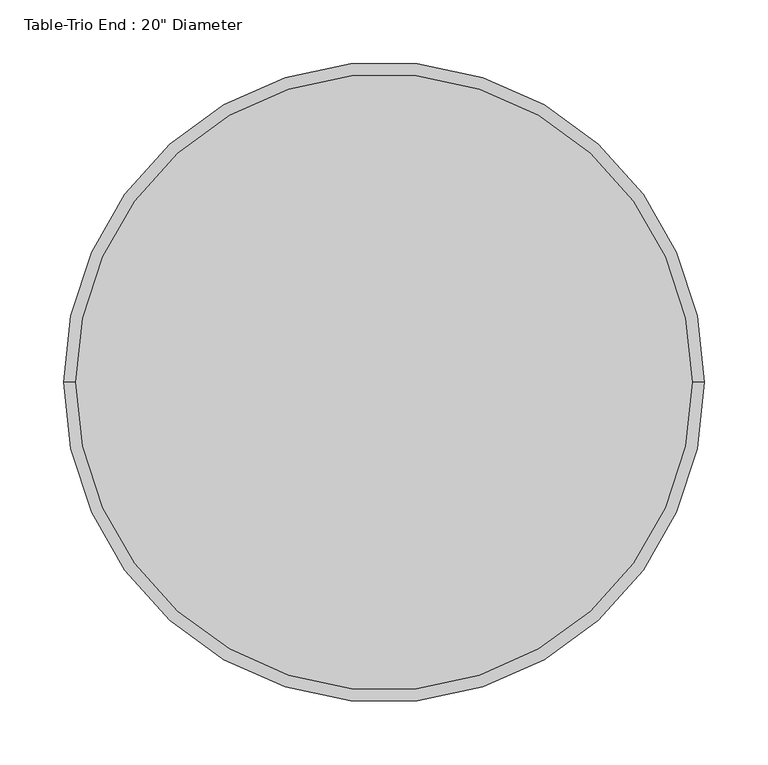
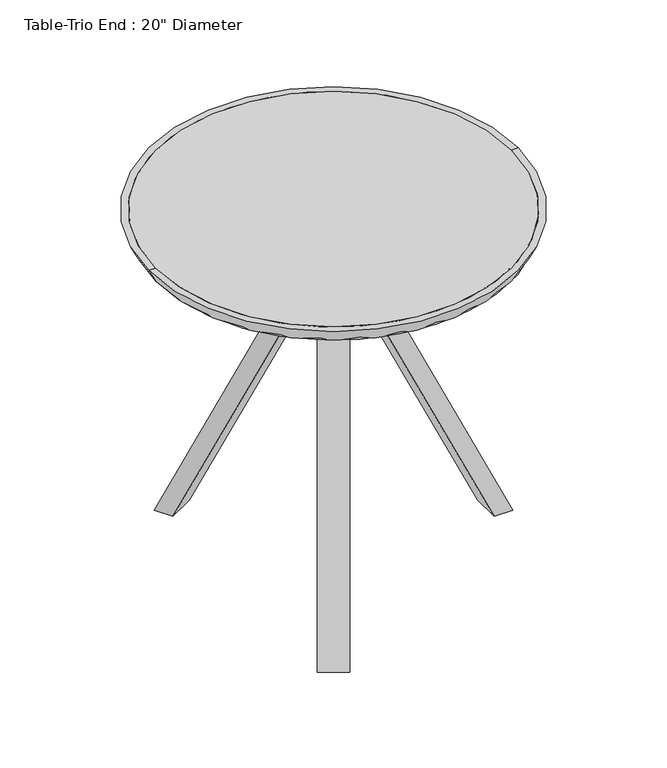
"""IFC4 building model written with IfcOpenShell, lengths in millimetres: furniture geometry."""

from ifc_helpers import new_model, si_unit, point, frame, frame_2d, origin, origin_2d, place, context, project, spatial, polyline, circle_curve, trimmed, segment, composite_curve, outline, extrude, source, transform, mapped, element, save
from ifc_brep_helpers import plane_surface, revolved_surface, advanced_brep


def furniture_9d41381f(model_context):
    return source(origin(), model_context, "Body", "SolidModel", [
        extrude(outline(composite_curve([segment(trimmed(circle_curve(origin_2d(), 241.3), [point((-241.3, 0.0))], [point((241.3, 0.0))], False, "CARTESIAN"), True, "CONTINUOUS"), segment(trimmed(circle_curve(origin_2d(), 241.3), [point((241.3, 0.0))], [point((-241.3, 0.0))], False, "CARTESIAN"), True, "CONTINUOUS")], self_intersect=False)), frame((0.0, 0.0, 482.6), z_axis=(0.0, 0.0, 1.0), x_axis=(1.0, 0.0, 0.0)), (0.0, 0.0, 1.0), 19.05),
        advanced_brep(
        [(241.3, 0.0, 482.6), (-241.3, 0.0, 482.6), (-241.3, 0.0, 501.65), (241.3, 0.0, 501.65), (250.825, 0.0, 501.65), (-250.825, 0.0, 501.65)],
        [
            (0, 1, circle_curve(frame((0.0, 0.0, 482.6), z_axis=(0.0, 0.0, -1.0), x_axis=(-1.0, 0.0, 0.0)), 241.3)),
            (1, 2),
            (2, 3, circle_curve(frame((0.0, 0.0, 501.65), z_axis=(0.0, 0.0, 1.0), x_axis=(-1.0, 0.0, 0.0)), 241.3)),
            (3, 0),
            (4, 5, circle_curve(frame((0.0, 0.0, 501.65), z_axis=(0.0, 0.0, -1.0), x_axis=(-1.0, 0.0, 0.0)), 250.825)),
            (5, 1),
            (0, 4),
            (2, 5),
            (4, 3),
            (1, 0, circle_curve(frame((0.0, 0.0, 482.6), z_axis=(0.0, 0.0, -1.0), x_axis=(1.0, 0.0, 0.0)), 241.3)),
            (3, 2, circle_curve(frame((0.0, 0.0, 501.65), z_axis=(0.0, 0.0, 1.0), x_axis=(1.0, 0.0, 0.0)), 241.3)),
            (5, 4, circle_curve(frame((0.0, 0.0, 501.65), z_axis=(0.0, 0.0, -1.0), x_axis=(1.0, 0.0, 0.0)), 250.825)),
        ],
        [
            revolved_surface(polyline([(-241.3, 0.0, 501.65), (-241.3, 0.0, 482.6)]), (0.0, 0.0, 0.0), (0.0, 0.0, 1.0)),
            revolved_surface(polyline([(-241.3, 0.0, 482.6), (-250.825, 0.0, 501.65)]), (0.0, 0.0, 0.0), (0.0, 0.0, 1.0)),
            plane_surface(frame((0.0, 0.0, 501.65), z_axis=(0.0, 0.0, 1.0), x_axis=(-1.0, 0.0, 0.0))),
            revolved_surface(polyline([(241.3, 0.0, 501.65), (241.3, 0.0, 482.6)]), (0.0, 0.0, 0.0), (0.0, 0.0, 1.0)),
            revolved_surface(polyline([(241.3, 0.0, 482.6), (250.825, 0.0, 501.65)]), (0.0, 0.0, 0.0), (0.0, 0.0, 1.0)),
            plane_surface(frame((0.0, 0.0, 501.65), z_axis=(0.0, 0.0, 1.0), x_axis=(1.0, 0.0, 0.0))),
        ],
        [
            (0, [[1, 2, 3, 4]]),
            (1, [[5, 6, -1, 7]]),
            (2, [[-3, 8, -5, 9]]),
            (3, [[10, -4, 11, -2]]),
            (4, [[12, -7, -10, -6]]),
            (5, [[-11, -9, -12, -8]]),
        ],
    ),
        extrude(outline(composite_curve([segment(polyline([(374.1964885, 32.5393466), (0.0, 207.0300348), (0.0, 232.3753669), (384.9309923, 52.8790974)]), True, "CONTINUOUS"), segment(trimmed(circle_curve(frame_2d((406.4, 98.9195329)), 50.8), [point((384.9309923, 52.8790974))], [point((457.2, 98.9195329))], True, "CARTESIAN"), True, "CONTINUOUS"), segment(polyline([(457.2, 98.9195329), (457.2, 154.8312035), (482.6, 154.8312035), (482.6, 101.6)]), True, "CONTINUOUS"), segment(trimmed(circle_curve(frame_2d((406.4, 101.6)), 76.2), [point((482.6, 101.6))], [point((374.1964885, 32.5393466))], False, "CARTESIAN"), True, "CONTINUOUS")], self_intersect=False)), frame((0.0, -19.05, 0.0), z_axis=(0.0, 1.0, 0.0), x_axis=(0.0, 0.0, 1.0)), (0.0, 0.0, 1.0), 38.1),
        extrude(outline(composite_curve([segment(trimmed(circle_curve(frame_2d((412.8801427, -76.2)), 76.2), [point((412.8801427, 0.0))], [point((481.9407961, -108.4035115))], False, "CARTESIAN"), True, "CONTINUOUS"), segment(polyline([(481.9407961, -108.4035115), (459.4443174, -156.6473658), (436.4240996, -145.9128619), (460.0533926, -95.2396796)]), True, "CONTINUOUS"), segment(trimmed(circle_curve(frame_2d((414.012957, -73.7706719)), 50.8), [point((460.0533926, -95.2396796))], [point((414.0129571, -22.9706718))], True, "CARTESIAN"), True, "CONTINUOUS"), segment(polyline([(414.0129571, -22.9706718), (-10.7114002, -22.9706719), (0.0, 0.0), (412.8801427, 0.0)]), True, "CONTINUOUS")], self_intersect=False)), frame((-120.0128014, 169.7682695, 0.0), z_axis=(0.8660254037844397, 0.4999999999999983, 0.0), x_axis=(0.2113091308703442, -0.36599815077065895, 0.9063077870366545)), (0.0, 0.0, 1.0), 38.1),
        extrude(outline(composite_curve([segment(trimmed(circle_curve(frame_2d((412.8801427, -76.2)), 76.2), [point((412.8801427, 0.0))], [point((481.9407961, -108.4035116))], False, "CARTESIAN"), True, "CONTINUOUS"), segment(polyline([(481.9407961, -108.4035116), (459.4443174, -156.6473658), (436.4240996, -145.9128619), (460.0533926, -95.2396796)]), True, "CONTINUOUS"), segment(trimmed(circle_curve(frame_2d((414.012957, -73.7706719)), 50.8), [point((460.0533926, -95.2396796))], [point((414.0129571, -22.9706718))], True, "CARTESIAN"), True, "CONTINUOUS"), segment(polyline([(414.0129571, -22.9706718), (-10.7114002, -22.9706719), (0.0, 0.0), (412.8801427, 0.0)]), True, "CONTINUOUS")], self_intersect=False)), frame((-87.0172335, -188.8182695, 0.0), z_axis=(-0.8660254037844366, 0.5000000000000038, 0.0), x_axis=(0.21130913087034656, 0.3659981507706578, 0.9063077870366544)), (0.0, 0.0, 1.0), 38.1),
        extrude(outline(composite_curve([segment(trimmed(circle_curve(origin_2d(), 31.7871474), [point((-31.7871474, 0.0))], [point((31.7871474, 0.0))], False, "CARTESIAN"), True, "CONTINUOUS"), segment(trimmed(circle_curve(origin_2d(), 31.7871474), [point((31.7871474, 0.0))], [point((-31.7871474, 0.0))], False, "CARTESIAN"), True, "CONTINUOUS")], self_intersect=False)), frame((0.0, 0.0, 381.0), z_axis=(0.0, 0.0, 1.0), x_axis=(1.0, 0.0, 0.0)), (0.0, 0.0, 1.0), 50.8),
    ])


if __name__ == "__main__":
    model = new_model("IFC4")
    model_context = context("Model", 3, world=origin())
    ifc_project = project(units=[si_unit("LENGTHUNIT", "METRE", prefix="MILLI")], contexts=[model_context])
    site = spatial("IfcSite", under=ifc_project)
    building = spatial("IfcBuilding", under=site)
    placement = place(None, origin())
    furniture_shape = furniture_9d41381f(model_context)
    element("IfcFurniture", 1, ObjectType="Table-Trio End : 20\" Diameter", at=placement, inside=building, context=model_context, shape_type="MappedRepresentation", body=[
        mapped(furniture_shape, transform((0.0, 0.0, 0.0), x_axis=(1.0, 0.0, 0.0), y_axis=(0.0, 1.0, 0.0), z_axis=(0.0, 0.0, 1.0))),
    ])
    save(model, "model.ifc")

# Revit data of these elements
# Type "Table-Trio End : 20\" Diameter"
#   Assembly Code = "E2020200"
#   Base and Trim Material = Wood - Birch
#   Table Top Material = Laminate - Ivory,Matte
#   Default Elevation = 0
# Element 1 (IfcFurniture, "Table-Trio End : 20\" Diameter")
#   Materials on its faces: "Wood - Birch", "Laminate - Ivory,Matte"
# Materials
#   "Wood - Birch": colour RGB 230 196 162, transparency 0
#   "Laminate - Ivory,Matte": colour RGB 247 247 239, transparency 0
